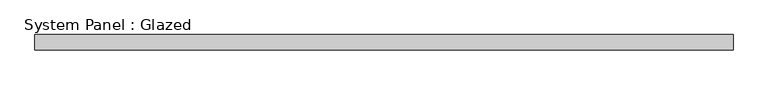
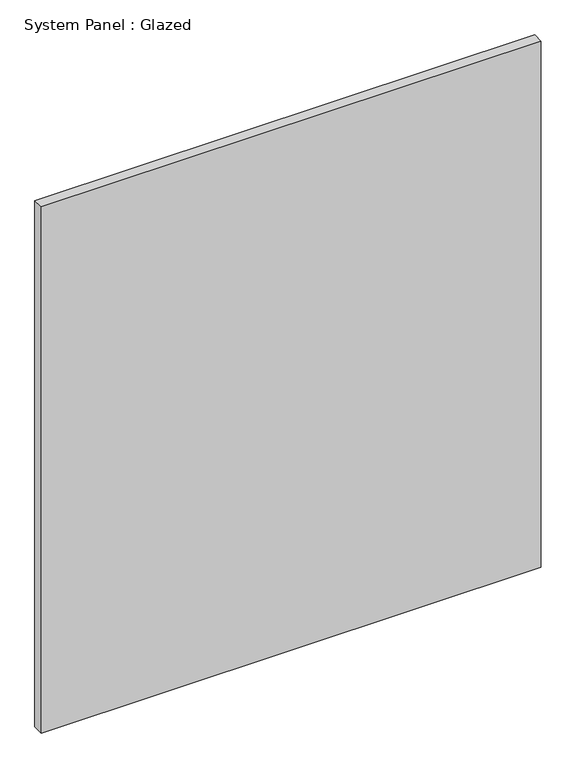
"""IFC4 building model written with IfcOpenShell, lengths in millimetres: plate geometry, System Panel : Glazed."""

from ifc_helpers import new_model, si_unit, origin, origin_with_axes, place, context, project, spatial, polyline, outline, extrude, source, transform, mapped, element, save


def system_panel_glazed_f332cf5d(model_context):
    return source(origin(), model_context, "Body", "SweptSolid", [
        extrude(outline(polyline([(581.0249999, 19.05), (-581.0249999, 19.05), (-581.0249999, 44.45), (581.0249999, 44.45), (581.0249999, 19.05)])), origin_with_axes(), (0.0, 0.0, 1.0), 1292.6724956),
    ])


if __name__ == "__main__":
    model = new_model("IFC4")
    model_context = context("Model", 3, world=origin())
    ifc_project = project(units=[si_unit("LENGTHUNIT", "METRE", prefix="MILLI")], contexts=[model_context])
    site = spatial("IfcSite", under=ifc_project)
    building = spatial("IfcBuilding", under=site)
    placement = place(None, origin())
    system_panel_glazed_shape = system_panel_glazed_f332cf5d(model_context)
    element("IfcPlate", 1, ObjectType="System Panel : Glazed", at=placement, inside=building, context=model_context, shape_type="MappedRepresentation", body=[
        mapped(system_panel_glazed_shape, transform((0.0, 0.0, 0.0), x_axis=(1.0, 0.0, 0.0), y_axis=(0.0, 1.0, 0.0), z_axis=(0.0, 0.0, 1.0))),
    ])
    save(model, "model.ifc")

# Revit data of these elements
# Type "System Panel : Glazed"
#   Construction Type Id = "GSP4R"
#   Analytic Construction = "1/8 in Pilkington single glazing"
#   Visual Light Transmittance = 0.9
#   Solar Heat Gain Coefficient = 0.86
#   Heat Transfer Coefficient (U) = 1.18115 BTU/(h·ft²·°F)
#   Define Thermal Properties by = 1
# Element 1 (IfcPlate, "System Panel : Glazed")
#   Materials on its faces: "Glass"
# Materials
#   "Glass": class "Glass", colour RGB 0 128 192, transparency 0.75, Description = "Soda Lime Glass", Cost = 0
